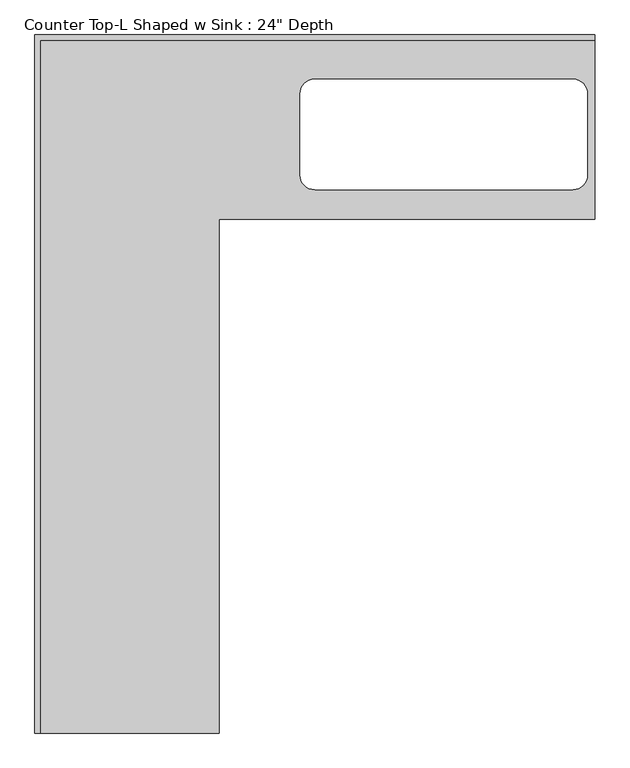
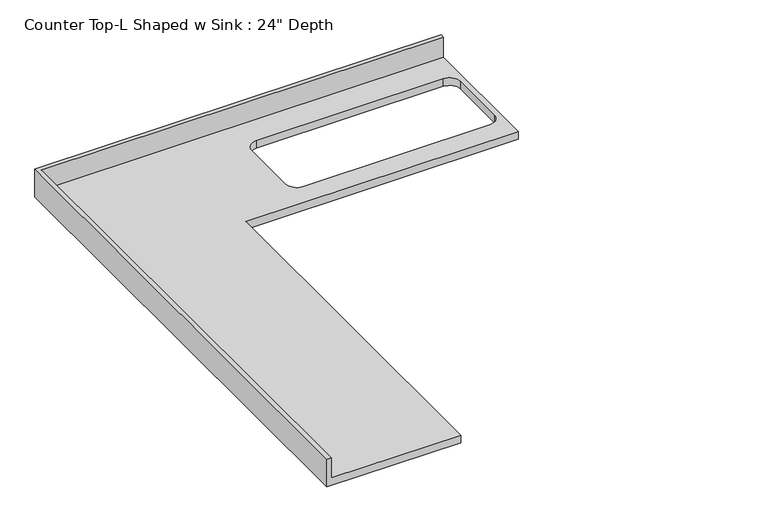
"""IFC4 building model written with IfcOpenShell, lengths in millimetres: furniture geometry."""

from ifc_helpers import new_model, si_unit, frame, origin, place, context, project, spatial, polyline, circle_curve, source, transform, mapped, element, save
from ifc_brep_helpers import plane_surface, revolved_surface, advanced_brep


def furniture_2f8694d0(model_context):
    return source(origin(), model_context, "Body", "AdvancedBrep", [
        advanced_brep(
        [(-565.4622951, -2404.8854158, 914.4), (-565.4622951, -635.0, 914.4), (729.9377049, -635.0, 914.4), (729.9377049, -19.05, 914.4), (-1181.4122951, -19.05, 914.4), (-1181.4122951, -2404.8854158, 914.4), (653.7377049, -152.4, 914.4), (704.5377049, -203.2, 914.4), (704.5377049, -482.6, 914.4), (653.7377049, -533.4, 914.4), (-235.2622951, -533.4, 914.4), (-286.0622951, -482.6, 914.4), (-286.0622951, -203.2, 914.4), (-235.2622951, -152.4, 914.4), (729.9377049, 0.0, 876.3), (729.9377049, -635.0, 876.3), (-565.4622951, -635.0, 876.3), (-565.4622951, -2404.8854158, 876.3), (-1200.4622951, -2404.8854158, 876.3), (-1200.4622951, 0.0, 876.3), (653.7377049, -152.4, 876.3), (-235.2622951, -152.4, 876.3), (-286.0622951, -203.2, 876.3), (-286.0622951, -482.6, 876.3), (-235.2622951, -533.4, 876.3), (653.7377049, -533.4, 876.3), (704.5377049, -482.6, 876.3), (704.5377049, -203.2, 876.3), (-1200.4622951, 0.0, 1016.0), (729.9377049, 0.0, 1016.0), (-1200.4622951, -2404.8854158, 1016.0), (-1181.4122951, -2404.8854158, 1016.0), (729.9377049, -19.05, 1016.0), (-1181.4122951, -19.05, 1016.0)],
        [
            (0, 1),
            (1, 2),
            (2, 3),
            (3, 4),
            (4, 5),
            (5, 0),
            (6, 7, circle_curve(frame((653.7377049, -203.2, 914.4), z_axis=(0.0, 0.0, -1.0), x_axis=(1.0, 0.0, 0.0)), 50.8)),
            (7, 8),
            (8, 9, circle_curve(frame((653.7377049, -482.6, 914.4), z_axis=(0.0, 0.0, -1.0), x_axis=(1.0, 0.0, 0.0)), 50.8)),
            (9, 10),
            (10, 11, circle_curve(frame((-235.2622951, -482.6, 914.4), z_axis=(0.0, 0.0, -1.0), x_axis=(1.0, 0.0, 0.0)), 50.8)),
            (11, 12),
            (12, 13, circle_curve(frame((-235.2622951, -203.2, 914.4), z_axis=(0.0, 0.0, -1.0), x_axis=(1.0, 0.0, 0.0)), 50.8)),
            (13, 6),
            (14, 15),
            (15, 16),
            (16, 17),
            (17, 18),
            (18, 19),
            (19, 14),
            (20, 21),
            (21, 22, circle_curve(frame((-235.2622951, -203.2, 876.3), z_axis=(0.0, 0.0, 1.0), x_axis=(1.0, 0.0, 0.0)), 50.8)),
            (22, 23),
            (23, 24, circle_curve(frame((-235.2622951, -482.6, 876.3), z_axis=(0.0, 0.0, 1.0), x_axis=(1.0, 0.0, 0.0)), 50.8)),
            (24, 25),
            (25, 26, circle_curve(frame((653.7377049, -482.6, 876.3), z_axis=(0.0, 0.0, 1.0), x_axis=(1.0, 0.0, 0.0)), 50.8)),
            (26, 27),
            (27, 20, circle_curve(frame((653.7377049, -203.2, 876.3), z_axis=(0.0, 0.0, 1.0), x_axis=(1.0, 0.0, 0.0)), 50.8)),
            (19, 28),
            (28, 29),
            (29, 14),
            (18, 30),
            (30, 28),
            (17, 0),
            (5, 31),
            (31, 30),
            (16, 1),
            (15, 2),
            (29, 32),
            (32, 3),
            (6, 20),
            (27, 7),
            (26, 8),
            (25, 9),
            (24, 10),
            (23, 11),
            (22, 12),
            (21, 13),
            (31, 33),
            (33, 32),
            (33, 4),
        ],
        [
            plane_surface(frame((-1200.4622951, 0.0, 914.4), z_axis=(0.0, 0.0, 1.0), x_axis=(-1.0, 0.0, 0.0))),
            plane_surface(frame((-1200.4622951, 0.0, 876.3), z_axis=(0.0, 0.0, -1.0), x_axis=(1.0, 0.0, 0.0))),
            plane_surface(frame((729.9377049, 0.0, 914.4), z_axis=(0.0, 1.0, 0.0), x_axis=(0.0, 0.0, -1.0))),
            plane_surface(frame((-1200.4622951, 0.0, 914.4), z_axis=(-1.0, 0.0, 0.0), x_axis=(0.0, 0.0, -1.0))),
            plane_surface(frame((-1200.4622951, -2404.8854158, 914.4), z_axis=(0.0, -1.0, 0.0), x_axis=(0.0, 0.0, -1.0))),
            plane_surface(frame((-565.4622951, -2404.8854158, 914.4), z_axis=(1.0, 0.0, 0.0), x_axis=(0.0, 0.0, -1.0))),
            plane_surface(frame((-565.4622951, -635.0, 914.4), z_axis=(0.0, -1.0, 0.0), x_axis=(0.0, 0.0, -1.0))),
            plane_surface(frame((729.9377049, -635.0, 914.4), z_axis=(1.0, 0.0, 0.0), x_axis=(0.0, 0.0, -1.0))),
            revolved_surface(polyline([(704.5377049, -203.2, 876.3), (704.5377049, -203.2, 914.4)]), (653.7377049, -203.2, 0.0), (0.0, 0.0, -1.0)),
            plane_surface(frame((704.5377049, -203.2, 914.4), z_axis=(-1.0, 0.0, 0.0), x_axis=(0.0, 0.0, -1.0))),
            revolved_surface(polyline([(704.5377049, -482.6, 876.3), (704.5377049, -482.6, 914.4)]), (653.7377049, -482.6, 0.0), (0.0, 0.0, -1.0)),
            plane_surface(frame((653.7377049, -533.4, 914.4), z_axis=(0.0, 1.0, 0.0), x_axis=(0.0, 0.0, -1.0))),
            revolved_surface(polyline([(-184.4622951, -482.6, 876.3), (-184.4622951, -482.6, 914.4)]), (-235.2622951, -482.6, 0.0), (0.0, 0.0, -1.0)),
            plane_surface(frame((-286.0622951, -482.6, 914.4), z_axis=(1.0, 0.0, 0.0), x_axis=(0.0, 0.0, -1.0))),
            revolved_surface(polyline([(-184.4622951, -203.2, 876.3), (-184.4622951, -203.2, 914.4)]), (-235.2622951, -203.2, 0.0), (0.0, 0.0, -1.0)),
            plane_surface(frame((-235.2622951, -152.4, 914.4), z_axis=(0.0, -1.0, 0.0), x_axis=(0.0, 0.0, -1.0))),
            plane_surface(frame((-1200.4622951, 0.0, 1016.0), z_axis=(0.0, 0.0, 1.0), x_axis=(0.0, -1.0, 0.0))),
            plane_surface(frame((-1200.4622951, -19.05, 1016.0), z_axis=(0.0, -1.0, 0.0), x_axis=(0.0, 0.0, -1.0))),
            plane_surface(frame((-1181.4122951, -2404.8854158, 1016.0), z_axis=(1.0, 0.0, 0.0), x_axis=(0.0, 0.0, -1.0))),
        ],
        [
            (0, [[1, 2, 3, 4, 5, 6], [7, 8, 9, 10, 11, 12, 13, 14]]),
            (1, [[15, 16, 17, 18, 19, 20], [21, 22, 23, 24, 25, 26, 27, 28]]),
            (2, [[-20, 29, 30, 31]]),
            (3, [[-19, 32, 33, -29]]),
            (4, [[-32, -18, 34, -6, 35, 36]]),
            (5, [[-1, -34, -17, 37]]),
            (6, [[-2, -37, -16, 38]]),
            (7, [[-15, -31, 39, 40, -3, -38]]),
            (8, [[-7, 41, -28, 42]]),
            (9, [[-8, -42, -27, 43]]),
            (10, [[-9, -43, -26, 44]]),
            (11, [[-10, -44, -25, 45]]),
            (12, [[-11, -45, -24, 46]]),
            (13, [[-12, -46, -23, 47]]),
            (14, [[-13, -47, -22, 48]]),
            (15, [[-14, -48, -21, -41]]),
            (16, [[-33, -36, 49, 50, -39, -30]]),
            (17, [[-40, -50, 51, -4]]),
            (18, [[-49, -35, -5, -51]]),
        ],
    ),
    ])


if __name__ == "__main__":
    model = new_model("IFC4")
    model_context = context("Model", 3, world=origin())
    ifc_project = project(units=[si_unit("LENGTHUNIT", "METRE", prefix="MILLI")], contexts=[model_context])
    site = spatial("IfcSite", under=ifc_project)
    building = spatial("IfcBuilding", under=site)
    placement = place(None, origin())
    furniture_shape = furniture_2f8694d0(model_context)
    element("IfcFurniture", 1, ObjectType="Counter Top-L Shaped w Sink : 24\" Depth", at=placement, inside=building, context=model_context, shape_type="MappedRepresentation", body=[
        mapped(furniture_shape, transform((0.0, 0.0, 0.0), x_axis=(1.0, 0.0, 0.0), y_axis=(0.0, 1.0, 0.0), z_axis=(0.0, 0.0, 1.0))),
    ])
    save(model, "model.ifc")

# Revit data of these elements
# Type "Counter Top-L Shaped w Sink : 24\" Depth"
#   Assembly Code = "C1030400"
#   Counter Thickness = 0' - 1 1/2"
#   Depth = 2' - 1"
#   Height = 3' - 0"
#   Length - Leg 1 [instance default] = 8' - 0"
#   Length - Leg 2 [instance default] = 6' - 0"
#   Sink Location [instance default] = 3' - 0"
#   Sink Location To Wall [instance default] = 0' - 6"
#   Sink Opening Depth [instance default] = 1' - 3"
#   Sink Opening Width [instance default] = 3' - 3"
#   Counter Top Material = none
#   Default Elevation = 0
# Element 1 (IfcFurniture, "Counter Top-L Shaped w Sink : 24\" Depth")
#   Length - Leg 1 = 6' - 4"
#   Length - Leg 2 = 7' - 10.68053"
#   Materials on its faces: "Counter Top"
# Materials
#   "Counter Top": class "Wood", colour RGB 226 177 128, transparency 0
